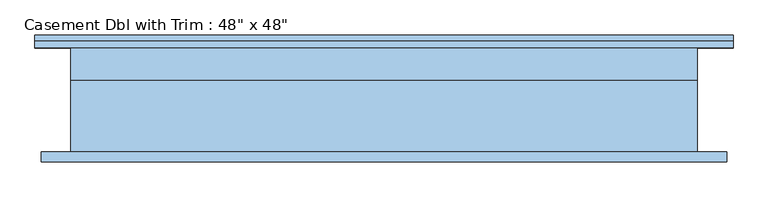
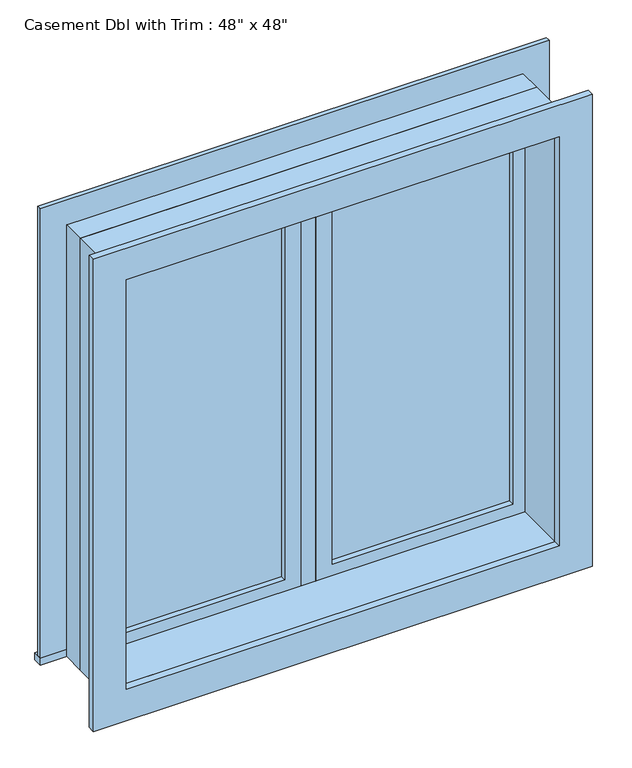
"""IFC4 building model written with IfcOpenShell, lengths in millimetres: window geometry."""

from ifc_helpers import new_model, si_unit, frame, origin, place, context, project, spatial, polyline, outline, extrude, source, transform, mapped, element, save


def window_0862ab64(model_context):
    return source(origin(), model_context, "Body", "SweptSolid", [
        extrude(outline(polyline([(63.5, 85.725), (546.1, 85.725), (546.1, 73.025), (63.5, 73.025), (63.5, 85.725)])), frame((0.0, 0.0, 977.9), z_axis=(0.0, 0.0, 1.0), x_axis=(1.0, 0.0, 0.0)), (0.0, 0.0, 1.0), 1092.2),
        extrude(outline(polyline([(2114.55, 19.05), (933.45, 19.05), (933.45, 590.55), (2114.55, 590.55), (2114.55, 19.05)]), holes=[polyline([(2070.1, 63.5), (2070.1, 546.1), (977.9, 546.1), (977.9, 63.5), (2070.1, 63.5)])]), frame((0.0, 57.15, 0.0), z_axis=(0.0, 1.0, 0.0), x_axis=(0.0, 0.0, 1.0)), (0.0, 0.0, 1.0), 44.45),
        extrude(outline(polyline([(19.05, 57.15), (-19.05, 57.15), (-19.05, 120.65), (19.05, 120.65), (19.05, 57.15)])), frame((0.0, 0.0, 933.45), z_axis=(0.0, 0.0, 1.0), x_axis=(1.0, 0.0, 0.0)), (0.0, 0.0, 1.0), 1181.1),
        extrude(outline(polyline([(-679.45, 146.05), (679.45, 146.05), (679.45, 120.65), (-679.45, 120.65), (-679.45, 146.05)])), frame((0.0, 0.0, 914.4), z_axis=(0.0, 0.0, 1.0), x_axis=(1.0, 0.0, 0.0)), (0.0, 0.0, 1.0), 19.05),
        extrude(outline(polyline([(2114.55, -590.55), (2114.55, 590.55), (933.45, 590.55), (933.45, 679.45), (2203.45, 679.45), (2203.45, -679.45), (933.45, -679.45), (933.45, -590.55), (2114.55, -590.55)])), frame((0.0, 120.65, 0.0), z_axis=(0.0, 1.0, 0.0), x_axis=(0.0, 0.0, 1.0)), (0.0, 0.0, 1.0), 12.7),
        extrude(outline(polyline([(2190.75, 666.75), (2190.75, -666.75), (857.25, -666.75), (857.25, 666.75), (2190.75, 666.75)]), holes=[polyline([(2101.85, 577.85), (946.15, 577.85), (946.15, -577.85), (2101.85, -577.85), (2101.85, 577.85)])]), frame((0.0, -101.6, 0.0), z_axis=(0.0, 1.0, 0.0), x_axis=(0.0, 0.0, 1.0)), (0.0, 0.0, 1.0), 19.05),
        extrude(outline(polyline([(-63.5, 73.025), (-546.1, 73.025), (-546.1, 85.725), (-63.5, 85.725), (-63.5, 73.025)])), frame((0.0, 0.0, 977.9), z_axis=(0.0, 0.0, 1.0), x_axis=(1.0, 0.0, 0.0)), (0.0, 0.0, 1.0), 1092.2),
        extrude(outline(polyline([(2114.55, -590.55), (933.45, -590.55), (933.45, -19.05), (2114.55, -19.05), (2114.55, -590.55)]), holes=[polyline([(2070.1, -546.1), (2070.1, -63.5), (977.9, -63.5), (977.9, -546.1), (2070.1, -546.1)])]), frame((0.0, 57.15, 0.0), z_axis=(0.0, 1.0, 0.0), x_axis=(0.0, 0.0, 1.0)), (0.0, 0.0, 1.0), 44.45),
        extrude(outline(polyline([(2133.6, -609.6), (914.4, -609.6), (914.4, 609.6), (2133.6, 609.6), (2133.6, -609.6)]), holes=[polyline([(2101.85, -577.85), (2101.85, 577.85), (946.15, 577.85), (946.15, -577.85), (2101.85, -577.85)])]), frame((0.0, -82.55, 0.0), z_axis=(0.0, 1.0, 0.0), x_axis=(0.0, 0.0, 1.0)), (0.0, 0.0, 1.0), 139.7),
        extrude(outline(polyline([(2133.6, 609.6), (2133.6, -609.6), (914.4, -609.6), (914.4, 609.6), (2133.6, 609.6)]), holes=[polyline([(2114.55, 590.55), (933.45, 590.55), (933.45, -590.55), (2114.55, -590.55), (2114.55, 590.55)])]), frame((0.0, 57.15, 0.0), z_axis=(0.0, 1.0, 0.0), x_axis=(0.0, 0.0, 1.0)), (0.0, 0.0, 1.0), 63.5),
    ])


if __name__ == "__main__":
    model = new_model("IFC4")
    model_context = context("Model", 3, world=origin())
    ifc_project = project(units=[si_unit("LENGTHUNIT", "METRE", prefix="MILLI")], contexts=[model_context])
    site = spatial("IfcSite", under=ifc_project)
    building = spatial("IfcBuilding", under=site)
    placement = place(None, origin())
    window_shape = window_0862ab64(model_context)
    element("IfcWindow", 1, ObjectType="Casement Dbl with Trim : 48\" x 48\"", at=placement, inside=building, context=model_context, shape_type="MappedRepresentation", body=[
        mapped(window_shape, transform((0.0, 0.0, 0.0), x_axis=(1.0, 0.0, 0.0), y_axis=(0.0, 1.0, 0.0), z_axis=(0.0, 0.0, 1.0))),
    ])
    save(model, "model.ifc")

# Revit data of these elements
# Type "Casement Dbl with Trim : 48\" x 48\""
#   Type Mark = "27"
#   Construction Type Id = "GSP4R"
#   Assembly Code = "B2020100"
#   Analytic Construction = "1/8 in Pilkington single glazing"
#   Visual Light Transmittance = 0.9
#   Solar Heat Gain Coefficient = 0.78
#   Heat Transfer Coefficient (U) = 0.6496 BTU/(h·ft²·°F)
#   Height = 4' - 0"
#   Default Sill Height = 3' - 0"
#   Trim Projection - Ext. = 0' - 0 1/2"
#   Trim Projection - Int. = 0' - 0 3/4"
#   Trim Width - Exterior = 0' - 3 1/2"
#   Trim Width - Interior = 0' - 3 1/2"
#   Width = 4' - 0"
#   Window Inset = 0' - 0 3/4"
#   Define Thermal Properties by = 1
#   Glass Pane Material = Glass
#   Sash Material = Sash
#   Trim Exterior Material = Trim
#   Trim Interior Material = Trim
#   Wall Closure = (empty or 0)
# Element 1 (IfcWindow, "Casement Dbl with Trim : 48\" x 48\"")
#   Materials on its faces: "Sash", "Trim", "Glass"
# Materials
#   "Glass": class "Glass", colour RGB 0 128 192, transparency 0.75, Description = "Soda Lime Glass", Cost = 0
#   "Sash": class "Wood", colour RGB 224 178 126, transparency 0
#   "Trim": class "Wood", colour RGB 224 178 126, transparency 0
